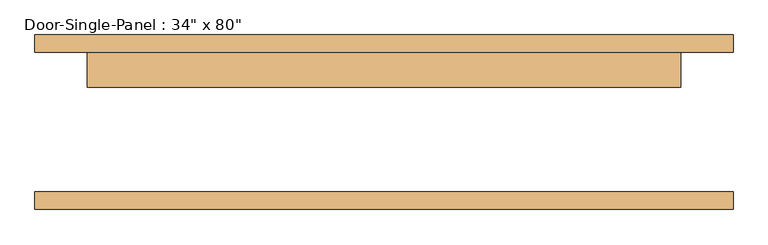
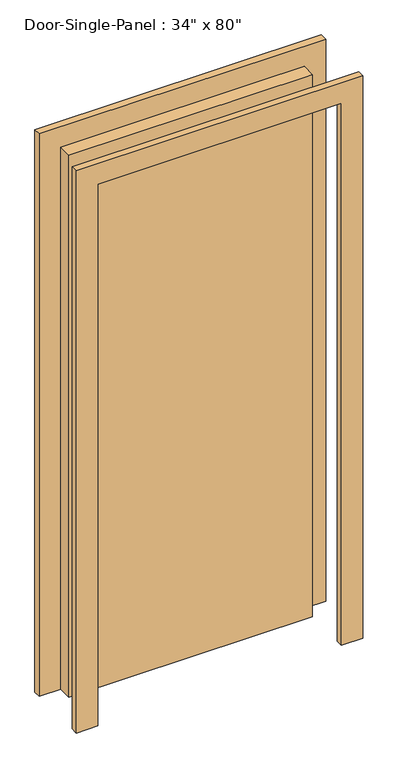
"""IFC4 building model written with IfcOpenShell, lengths in millimetres: door geometry."""

from ifc_helpers import new_model, si_unit, frame, origin, origin_with_axes, place, context, project, spatial, polyline, outline, extrude, source, transform, mapped, element, save


def door_10fd3a06(model_context):
    return source(origin(), model_context, "Body", "SweptSolid", [
        extrude(outline(polyline([(431.8, 50.8), (-431.8, 50.8), (-431.8, 101.6), (431.8, 101.6), (431.8, 50.8)])), origin_with_axes(), (0.0, 0.0, 1.0), 2032.0),
        extrude(outline(polyline([(2108.2, -508.0), (0.0, -508.0), (0.0, -431.8), (2032.0, -431.8), (2032.0, 431.8), (0.0, 431.8), (0.0, 508.0), (2108.2, 508.0), (2108.2, -508.0)])), frame((0.0, 101.6, 0.0), z_axis=(0.0, 1.0, 0.0), x_axis=(0.0, 0.0, 1.0)), (0.0, 0.0, 1.0), 25.4),
        extrude(outline(polyline([(2108.2, 508.0), (2108.2, -508.0), (0.0, -508.0), (0.0, -431.8), (2032.0, -431.8), (2032.0, 431.8), (0.0, 431.8), (0.0, 508.0), (2108.2, 508.0)])), frame((0.0, -127.0, 0.0), z_axis=(0.0, 1.0, 0.0), x_axis=(0.0, 0.0, 1.0)), (0.0, 0.0, 1.0), 25.4),
    ])


if __name__ == "__main__":
    model = new_model("IFC4")
    model_context = context("Model", 3, world=origin())
    ifc_project = project(units=[si_unit("LENGTHUNIT", "METRE", prefix="MILLI")], contexts=[model_context])
    site = spatial("IfcSite", under=ifc_project)
    building = spatial("IfcBuilding", under=site)
    placement = place(None, origin())
    door_shape = door_10fd3a06(model_context)
    element("IfcDoor", 1, ObjectType="Door-Single-Panel : 34\" x 80\"", at=placement, inside=building, context=model_context, shape_type="MappedRepresentation", body=[
        mapped(door_shape, transform((0.0, 0.0, 0.0), x_axis=(1.0, 0.0, 0.0), y_axis=(0.0, 1.0, 0.0), z_axis=(0.0, 0.0, 1.0))),
    ])
    save(model, "model.ifc")

# Revit data of these elements
# Type "Door-Single-Panel : 34\" x 80\""
#   Type Mark = "8"
#   Construction Type Id = "DOOR"
#   Assembly Code = "C1020300"
#   Analytic Construction = "Wooden"
#   Thickness = 0' - 2"
#   Thermal Resistance (R) = 2.5876 (h·ft²·°F)/BTU
#   Swing Angle [instance default] = 90.00°
#   Heat Transfer Coefficient (U) = 0.3865 BTU/(h·ft²·°F)
#   Height = 6' - 8"
#   Trim Projection Ext = 0' - 1"
#   Trim Projection Int = 0' - 1"
#   Trim Width = 0' - 3"
#   Width = 2' - 10"
#   Define Thermal Properties by = 1
#   Panel Material = Wood - Birch - Solid Stained Light Low Gloss
#   Trim Material = Roofing, EPDM Membrane
#   Visual Light Transmittance = 0
#   Solar Heat Gain Coefficient = 0
#   Function = (empty or 0)
#   Wall Closure = (empty or 0)
# Element 1 (IfcDoor, "Door-Single-Panel : 34\" x 80\"")
#   Materials on its faces: "Roofing, EPDM Membrane", "Wood - Birch - Solid Stained Light Low Gloss"
# Materials
#   "Wood - Birch - Solid Stained Light Low Gloss": class "Wood", colour RGB 210 159 95, transparency 0, Cost = 0
#   "Roofing, EPDM Membrane": class "Generic", colour RGB 127 127 127, transparency 0, Description = "EPDM roof membrane", Cost = 0
